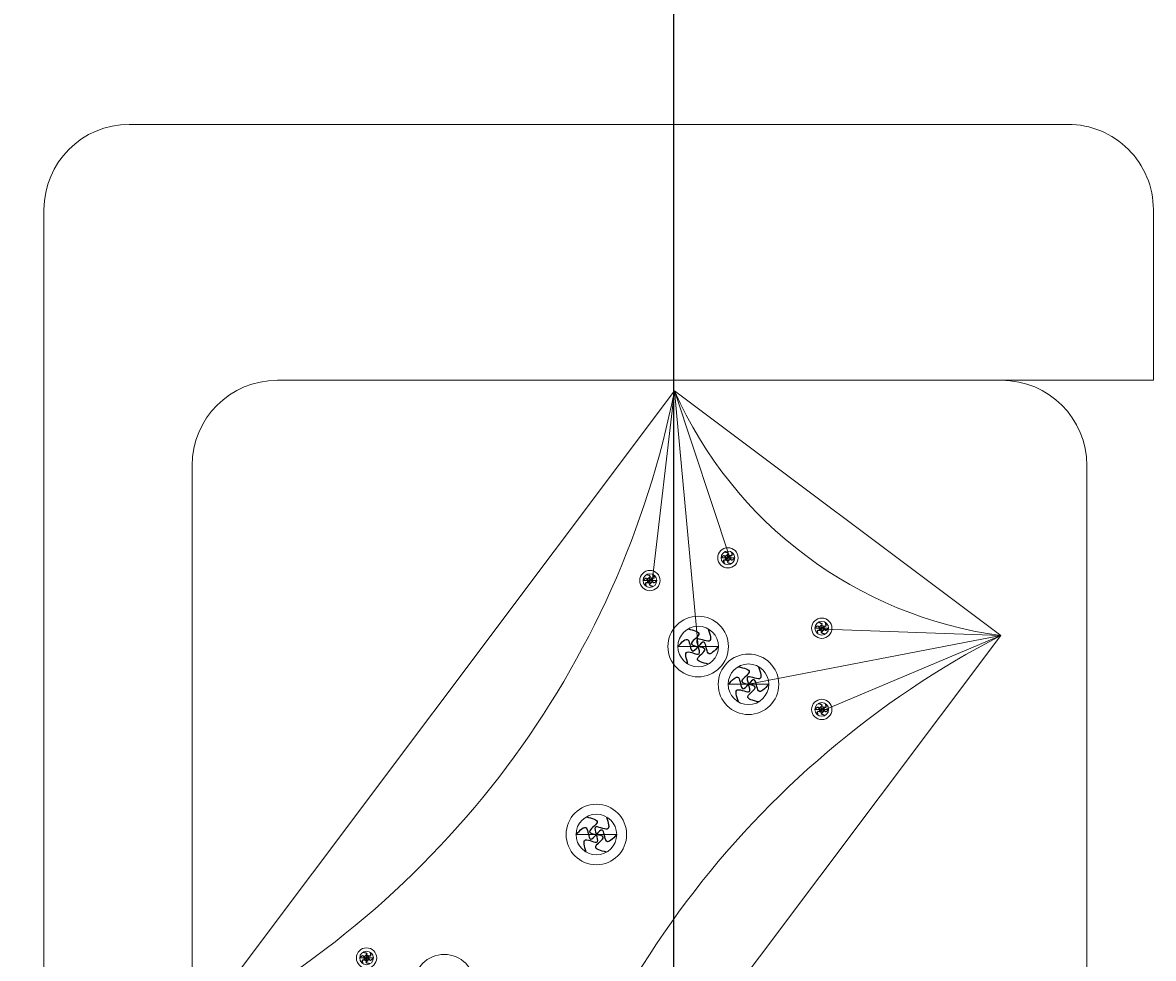
# Model space of a CAD drawing. Units: inches. Extents: x -61 to 1599, y -1316 to 257.
# Tile 27 of 204: x 388 to 415, y -873 to -851. Entities that reach past the tile are written whole.
import ezdxf

# ---------------------------------------------------------------- set-up
doc = ezdxf.new("R2010")
doc.units = ezdxf.units.IN
doc.header["$MEASUREMENT"] = 0
doc.layers.add('A-ANNO-DIMS', color=2, linetype='Continuous', lineweight=18)
doc.layers.add('FURNITURE', color=83, linetype='Continuous', lineweight=18)
doc.layers.add('FUR', color=83, linetype='Continuous')
doc.styles.get("Standard").update_dxf_attribs({"font": 'arial.ttf'})
doc.dimstyles.get("Standard").update_dxf_attribs({"dimtxt": 0.18, "dimasz": 0.18, "dimexe": 0.18, "dimexo": 0.0625, "dimgap": 0.09, "dimtad": 0, "dimtih": 1, "dimtoh": 1, "dimdec": 0, "dimzin": 0, "dimdsep": 46, "dimlunit": 3, "dimtxsty": 'Standard', "dimcen": 0.09, "dimadec": 0, "dimazin": 0, "dimtfac": 1, "dimtdec": 0, "dimtofl": 0, "dimtmove": 0, "dimatfit": 3, "dimfxl": 1, "dimtolj": 1, "dimtzin": 0, "dimarcsym": 0})

# ---------------------------------------------------------------- blocks, each defined once
blk = doc.blocks.new('*U186')
at = {"layer": 'FUR'}
blk.add_open_spline([(0.005, 0.08), (-0.03, 0.048), (-0.098, -0.015), (0.075, -0.018), (0.024, -0.063), (0.005, -0.08)], degree=3, knots=[0, 0, 0, 0, 0.0954578, 0.1898773, 0.2470677, 0.2470677, 0.2470677, 0.2470677], dxfattribs=at)
blk = doc.blocks.new('*U187')
at = {"layer": 'FUR', "transparency": 16777216}
for p, rotation in [((222.173, -79.977), 60), ((222.178, -80.056), 120), ((222.25, -80.092), 180), ((222.312, -79.968), 300), ((222.317, -80.048), 240)]:
    blk.add_blockref('*U186', p, dxfattribs=dict(at, rotation=rotation))
blk.add_blockref('*U186', (222.24, -79.932), dxfattribs=at)
blk = doc.blocks.new('*U196')
at = {"layer": 'FUR'}
blk.add_open_spline([(0.015, 0.238), (-0.088, 0.143), (-0.292, -0.045), (0.224, -0.053), (0.072, -0.187), (0.015, -0.238)], degree=3, knots=[0, 0, 0, 0, 0.2846533, 0.5662105, 0.736751, 0.736751, 0.736751, 0.736751], dxfattribs=at)
blk = doc.blocks.new('*U197')
at = {"layer": 'FUR', "transparency": 16777216}
blk.add_blockref('*U196', (662.716, -238.357), dxfattribs=at)
for p, rotation in [((662.929, -238.463), 300), ((662.517, -238.489), 60), ((662.531, -238.727), 120), ((662.944, -238.702), 240), ((662.745, -238.833), 180)]:
    blk.add_blockref('*U196', p, dxfattribs=dict(at, rotation=rotation))
blk = doc.blocks.new('*U190')
at = {"layer": 'FUR'}
blk.add_open_spline([(0.005, 0.08), (-0.03, 0.048), (-0.098, -0.015), (0.075, -0.018), (0.024, -0.063), (0.005, -0.08)], degree=3, knots=[0, 0, 0, 0, 0.0954578, 0.1898773, 0.2470677, 0.2470677, 0.2470677, 0.2470677], dxfattribs=at)
blk = doc.blocks.new('*U191')
at = {"layer": 'FUR', "transparency": 16777216}
for p, rotation in [((222.173, -79.977), 60), ((222.178, -80.056), 120), ((222.25, -80.092), 180), ((222.312, -79.968), 300), ((222.317, -80.048), 240)]:
    blk.add_blockref('*U190', p, dxfattribs=dict(at, rotation=rotation))
blk.add_blockref('*U190', (222.24, -79.932), dxfattribs=at)
blk = doc.blocks.new('*U209')
at = {"layer": 'FUR'}
blk.add_open_spline([(0.015, 0.238), (-0.088, 0.143), (-0.292, -0.045), (0.224, -0.053), (0.072, -0.187), (0.015, -0.238)], degree=3, knots=[0, 0, 0, 0, 0.2846533, 0.5662105, 0.736751, 0.736751, 0.736751, 0.736751], dxfattribs=at)
blk = doc.blocks.new('*U188')
at = {"layer": 'FUR', "transparency": 16777216}
blk.add_blockref('*U209', (662.716, -238.357), dxfattribs=at)
for p, rotation in [((662.929, -238.463), 300), ((662.517, -238.489), 60), ((662.531, -238.727), 120), ((662.944, -238.702), 240), ((662.745, -238.833), 180)]:
    blk.add_blockref('*U209', p, dxfattribs=dict(at, rotation=rotation))
blk = doc.blocks.new('*U208')
at = {"layer": 'FUR'}
blk.add_open_spline([(0.005, 0.08), (-0.03, 0.048), (-0.098, -0.015), (0.075, -0.018), (0.024, -0.063), (0.005, -0.08)], degree=3, knots=[0, 0, 0, 0, 0.0954578, 0.1898773, 0.2470677, 0.2470677, 0.2470677, 0.2470677], dxfattribs=at)
blk = doc.blocks.new('*U189')
at = {"layer": 'FUR', "transparency": 16777216}
for p, rotation in [((222.173, -79.977), 60), ((222.178, -80.056), 120), ((222.25, -80.092), 180), ((222.312, -79.968), 300), ((222.317, -80.048), 240)]:
    blk.add_blockref('*U208', p, dxfattribs=dict(at, rotation=rotation))
blk.add_blockref('*U208', (222.24, -79.932), dxfattribs=at)
blk = doc.blocks.new('*U192')
at = {"layer": 'FUR'}
blk.add_open_spline([(0.015, 0.238), (-0.088, 0.143), (-0.292, -0.045), (0.224, -0.053), (0.072, -0.187), (0.015, -0.238)], degree=3, knots=[0, 0, 0, 0, 0.2846533, 0.5662105, 0.736751, 0.736751, 0.736751, 0.736751], dxfattribs=at)
blk = doc.blocks.new('*U193')
at = {"layer": 'FUR', "transparency": 16777216}
blk.add_blockref('*U192', (662.716, -238.357), dxfattribs=at)
for p, rotation in [((662.929, -238.463), 300), ((662.517, -238.489), 60), ((662.531, -238.727), 120), ((662.944, -238.702), 240), ((662.745, -238.833), 180)]:
    blk.add_blockref('*U192', p, dxfattribs=dict(at, rotation=rotation))
blk = doc.blocks.new('*U204')
at = {"layer": 'FUR'}
blk.add_open_spline([(0.005, 0.08), (-0.03, 0.048), (-0.098, -0.015), (0.075, -0.018), (0.024, -0.063), (0.005, -0.08)], degree=3, knots=[0, 0, 0, 0, 0.0954578, 0.1898773, 0.2470677, 0.2470677, 0.2470677, 0.2470677], dxfattribs=at)
blk = doc.blocks.new('*U205')
at = {"layer": 'FUR', "transparency": 16777216}
for p, rotation in [((222.173, -79.977), 60), ((222.178, -80.056), 120), ((222.25, -80.092), 180), ((222.312, -79.968), 300), ((222.317, -80.048), 240)]:
    blk.add_blockref('*U204', p, dxfattribs=dict(at, rotation=rotation))
blk.add_blockref('*U204', (222.24, -79.932), dxfattribs=at)
blk = doc.blocks.new('*U206')
at = {"layer": 'FUR'}
blk.add_open_spline([(0.005, 0.08), (-0.03, 0.048), (-0.098, -0.015), (0.075, -0.018), (0.024, -0.063), (0.005, -0.08)], degree=3, knots=[0, 0, 0, 0, 0.0954578, 0.1898773, 0.2470677, 0.2470677, 0.2470677, 0.2470677], dxfattribs=at)
blk = doc.blocks.new('*U207')
at = {"layer": 'FUR', "transparency": 16777216}
for p, rotation in [((222.173, -79.977), 60), ((222.178, -80.056), 120), ((222.25, -80.092), 180), ((222.312, -79.968), 300), ((222.317, -80.048), 240)]:
    blk.add_blockref('*U206', p, dxfattribs=dict(at, rotation=rotation))
blk.add_blockref('*U206', (222.24, -79.932), dxfattribs=at)
blk = doc.blocks.new('SOFA-LOVESEAT')
for p, q in [((22.442, 54), (5.47, 54)), ((22.442, 54), (26, 54)), ((14.776, 53.751), (14.253, 49.285)), ((14.776, 53.751), (15.332, 47.757)), ((14.776, 53.751), (16.081, 49.817)), ((3.47, 8), (3.47, 52)), ((24.442, 52), (24.442, 32)), ((16.029, 49.837), (15.869, 49.837)), ((16.029, 49.837), (16.189, 49.837)), ((14.201, 49.305), (14.041, 49.305)), ((14.201, 49.305), (14.36, 49.305)), ((22.422, 48.013), (16.511, 46.872)), ((18.228, 48.187), (18.068, 48.187)), ((18.228, 48.187), (18.388, 48.187)), ((22.422, 48.013), (18.28, 48.167)), ((22.422, 48.013), (18.28, 46.263)), ((15.332, 47.757), (14.855, 47.757)), ((15.332, 47.757), (15.808, 47.757)), ((16.511, 46.872), (16.035, 46.872)), ((16.511, 46.872), (16.988, 46.872)), ((18.228, 46.282), (18.068, 46.282)), ((18.228, 46.282), (18.388, 46.282)), ((12.946, 43.35), (12.47, 43.35)), ((12.946, 43.35), (13.423, 43.35)), ((7.56, 40.455), (7.4, 40.455)), ((7.56, 40.455), (7.719, 40.455))]:
    blk.add_line(p, q)
blk.add_lwpolyline([(26, 6), (26, 2, -0.414214), (24, 0), (2, 0, -0.414214), (0, 2), (0, 58, -0.414213), (2, 60), (24, 60, -0.414214), (26, 58), (26, 54)], format="xyb")
blk.add_lwpolyline([(11.116, 32.948), (22.422, 48.013), (14.776, 53.751), (3.47, 38.686)], close=True)
for centre, radius in [((16.029, 49.837), 0.238), ((16.029, 49.837), 0.16), ((14.201, 49.305), 0.238), ((14.201, 49.305), 0.16), ((15.332, 47.757), 0.71), ((15.332, 47.757), 0.476), ((18.228, 48.187), 0.238), ((18.228, 48.187), 0.16), ((16.511, 46.872), 0.71), ((16.511, 46.872), 0.476), ((18.228, 46.282), 0.238), ((18.228, 46.282), 0.16), ((12.946, 43.35), 0.71), ((12.946, 43.35), 0.476), ((7.56, 40.455), 0.238), ((7.56, 40.455), 0.16), ((9.381, 39.828), 0.71)]:
    blk.add_circle(centre, radius)
for centre, radius, start, end in [((5.47, 52), 2, 90, 180), ((22.442, 52), 2, 0, 90), ((-6.541, 57.974), 21.731, 297.4317, 348.7956), ((23.745, 57.74), 9.816, 203.9742, 262.253), ((32.433, 28.726), 21.731, 117.4317, 168.7956)]:
    blk.add_arc(centre, radius, start, end)
at = {"xscale": -1, "rotation": 90.00003000000098}
for name, p in [('*U189', (-63.984, 272.082)), ('*U191', (-65.812, 271.55)), ('*U188', (-223.264, 710.487)), ('*U205', (-61.785, 270.431)), ('*U193', (-222.084, 709.602)), ('*U207', (-61.785, 268.527)), ('*U197', (-225.649, 706.08)), ('*U187', (-72.453, 262.7))]:
    blk.add_blockref(name, p, dxfattribs=at)
blk = doc.blocks.new('*D710')
at = {"layer": 'A-ANNO-DIMS', "color": 0, "lineweight": -2, "transparency": 16777216}
for p, q in [((319.703, -465.385), (319.703, -1315.725)), ((403.703, -465.385), (403.703, -1315.725)), ((319.883, -1315.545), (361.484, -1315.545)), ((403.523, -1315.545), (361.921, -1315.545))]:
    blk.add_line(p, q, dxfattribs=at)
at = {"layer": 'A-ANNO-DIMS', "color": 0, "transparency": 16777216}
for points in [[(319.883, -1315.515), (319.883, -1315.575), (319.703, -1315.545)], [(403.523, -1315.515), (403.523, -1315.575), (403.703, -1315.545)]]:
    blk.add_solid(points, dxfattribs=at)
at = {"layer": 'DEFPOINTS', "color": 0, "transparency": 16777216}
for p in [(319.703, -465.323), (403.703, -465.323), (403.703, -1315.545)]:
    blk.add_point(p, dxfattribs=at)
at = {"layer": 'A-ANNO-DIMS', "color": 0, "transparency": 16777216, "insert": (361.703, -1315.545), "char_height": 0.18, "attachment_point": 5}
blk.add_mtext('\\A1;84', dxfattribs=at)

msp = doc.modelspace()

# ---------------------------------------------------------------- block references
at = {"layer": 'FURNITURE'}
msp.add_blockref('SOFA-LOVESEAT', (388.9518, -913.0047), dxfattribs=at)

# ---------------------------------------------------------------- dimensions: what is measured, and where the dimension line sits
at = {"layer": 'A-ANNO-DIMS'}
dim = msp.add_linear_dim(base=(403.7028, -1315.5446), p1=(319.7028, -465.3229), p2=(403.7028, -465.3229), dimstyle='Standard', override={"dimdec": 0, "dimlfac": 1, "dimrnd": 0, "dimzin": 0, "dimdsep": 46, "dimlunit": 2}, dxfattribs=at)
dim.commit()
dim.dimension.update_dxf_attribs({"geometry": '*D710', "text_midpoint": (361.7028, -1315.5446)})

doc.saveas('drawing.dxf')
